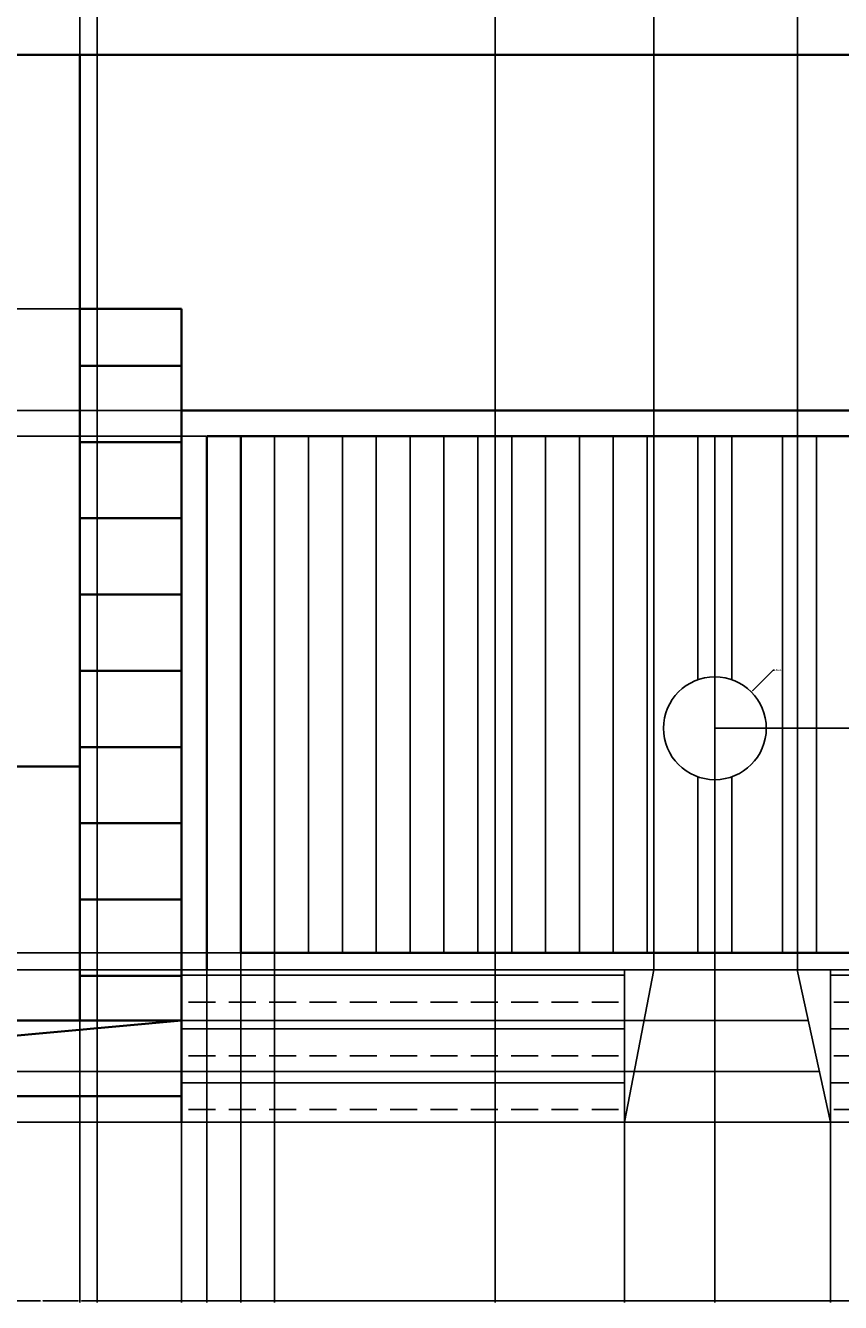
# Model space of a CAD drawing. Units: inches. Extents: x 2148 to 2587, y 1015 to 1466.
# Tile 2 of 7: x 2310 to 2406, y 1015 to 1166. Entities that reach past the tile are written whole.
import ezdxf

# ---------------------------------------------------------------- set-up
doc = ezdxf.new("R2010")
doc.units = ezdxf.units.IN
for name, color, linetype, lineweight in [('A-ANNO-DIMS', 2, 'Continuous', 18), ('A-DOOR', 3, 'Continuous', 25), ('A-ELEV', 7, 'Continuous', 35), ('A-FLOR-STRS', 2, 'Continuous', 25)]:
    doc.layers.add(name, color=color, linetype=linetype, lineweight=lineweight)
doc.styles.get("Standard").update_dxf_attribs({"font": 'arial.ttf'})
doc.dimstyles.get("Standard").update_dxf_attribs({"dimtxt": 0.18, "dimasz": 0.18, "dimexe": 0.18, "dimexo": 0.0625, "dimgap": 0.09, "dimtad": 0, "dimtih": 1, "dimtoh": 1, "dimdec": 4, "dimzin": 0, "dimdsep": 46, "dimtxsty": 'Standard', "dimcen": 0.09, "dimadec": 0, "dimazin": 0, "dimtfac": 1, "dimtdec": 4, "dimtofl": 0, "dimtmove": 0, "dimatfit": 3, "dimfxl": 1, "dimtolj": 1, "dimtzin": 0, "dimarcsym": 0})

# ---------------------------------------------------------------- blocks, each defined once
blk = doc.blocks.new('*D11')
at = {"layer": 'A-ANNO-DIMS', "color": 0, "lineweight": -2, "transparency": 16777216}
for p, q in [((2307.03, 1048.68), (2307.03, 1015.46)), ((2316.03, 1048.68), (2316.03, 1015.46)), ((2307.21, 1015.64), (2311.39, 1015.64)), ((2315.85, 1015.64), (2311.68, 1015.64))]:
    blk.add_line(p, q, dxfattribs=at)
at = {"layer": 'A-ANNO-DIMS', "color": 0, "transparency": 16777216}
for points in [[(2307.21, 1015.67), (2307.21, 1015.61), (2307.03, 1015.64)], [(2315.85, 1015.67), (2315.85, 1015.61), (2316.03, 1015.64)]]:
    blk.add_solid(points, dxfattribs=at)
at = {"layer": 'Defpoints', "color": 0, "transparency": 16777216}
for p in [(2307.03, 1048.74), (2316.03, 1048.74), (2316.03, 1015.64)]:
    blk.add_point(p, dxfattribs=at)
at = {"layer": 'A-ANNO-DIMS', "color": 0, "transparency": 16777216, "insert": (2311.53, 1015.64), "char_height": 0.18, "attachment_point": 5}
blk.add_mtext('\\A1;9', dxfattribs=at)
blk = doc.blocks.new('*D12')
at = {"layer": 'A-ANNO-DIMS', "color": 0, "lineweight": -2, "transparency": 16777216}
for p, q in [((2316.03, 1162.68), (2316.03, 1015.46)), ((2466.03, 1048.68), (2466.03, 1015.46)), ((2316.21, 1015.64), (2390.75, 1015.64)), ((2465.85, 1015.64), (2391.31, 1015.64))]:
    blk.add_line(p, q, dxfattribs=at)
at = {"layer": 'A-ANNO-DIMS', "color": 0, "transparency": 16777216}
for points in [[(2316.21, 1015.67), (2316.21, 1015.61), (2316.03, 1015.64)], [(2465.85, 1015.67), (2465.85, 1015.61), (2466.03, 1015.64)]]:
    blk.add_solid(points, dxfattribs=at)
at = {"layer": 'Defpoints', "color": 0, "transparency": 16777216}
for p in [(2316.03, 1162.74), (2466.03, 1048.74), (2466.03, 1015.64)]:
    blk.add_point(p, dxfattribs=at)
at = {"layer": 'A-ANNO-DIMS', "color": 0, "transparency": 16777216, "insert": (2391.03, 1015.64), "char_height": 0.18, "attachment_point": 5}
blk.add_mtext('\\A1;150', dxfattribs=at)
blk = doc.blocks.new('*D47')
at = {"layer": 'A-ANNO-DIMS', "color": 0, "lineweight": -2, "transparency": 16777216}
for p, q in [((2307.03, 1334.68), (2307.03, 1015.46)), ((2316.03, 1329.68), (2316.03, 1015.46)), ((2307.21, 1015.64), (2311.39, 1015.64)), ((2315.85, 1015.64), (2311.68, 1015.64))]:
    blk.add_line(p, q, dxfattribs=at)
at = {"layer": 'A-ANNO-DIMS', "color": 0, "transparency": 16777216}
for points in [[(2307.21, 1015.67), (2307.21, 1015.61), (2307.03, 1015.64)], [(2315.85, 1015.67), (2315.85, 1015.61), (2316.03, 1015.64)]]:
    blk.add_solid(points, dxfattribs=at)
at = {"layer": 'Defpoints', "color": 0, "transparency": 16777216}
for p in [(2307.03, 1334.74), (2316.03, 1329.74), (2316.03, 1015.64)]:
    blk.add_point(p, dxfattribs=at)
at = {"layer": 'A-ANNO-DIMS', "color": 0, "transparency": 16777216, "insert": (2311.53, 1015.64), "char_height": 0.18, "attachment_point": 5}
blk.add_mtext('\\A1;9', dxfattribs=at)
blk = doc.blocks.new('*D48')
at = {"layer": 'A-ANNO-DIMS', "color": 0, "lineweight": -2, "transparency": 16777216}
for p, q in [((2316.03, 1329.68), (2316.03, 1015.46)), ((2318.08, 1174.68), (2318.08, 1015.46)), ((2316.21, 1015.64), (2316.73, 1015.64)), ((2317.9, 1015.64), (2317.38, 1015.64))]:
    blk.add_line(p, q, dxfattribs=at)
at = {"layer": 'A-ANNO-DIMS', "color": 0, "transparency": 16777216}
for points in [[(2316.21, 1015.67), (2316.21, 1015.61), (2316.03, 1015.64)], [(2317.9, 1015.67), (2317.9, 1015.61), (2318.08, 1015.64)]]:
    blk.add_solid(points, dxfattribs=at)
at = {"layer": 'Defpoints', "color": 0, "transparency": 16777216}
for p in [(2316.03, 1329.74), (2318.08, 1174.74), (2318.08, 1015.64)]:
    blk.add_point(p, dxfattribs=at)
at = {"layer": 'A-ANNO-DIMS', "color": 0, "transparency": 16777216, "insert": (2317.06, 1015.64), "char_height": 0.18, "attachment_point": 5}
blk.add_mtext('\\A1;2.05', dxfattribs=at)
blk = doc.blocks.new('*D49')
at = {"layer": 'A-ANNO-DIMS', "color": 0, "lineweight": -2, "transparency": 16777216}
for p, q in [((2318.08, 1174.68), (2318.08, 1015.46)), ((2365.07, 1174.68), (2365.07, 1015.46)), ((2318.26, 1015.64), (2341.18, 1015.64)), ((2364.89, 1015.64), (2341.97, 1015.64))]:
    blk.add_line(p, q, dxfattribs=at)
at = {"layer": 'A-ANNO-DIMS', "color": 0, "transparency": 16777216}
for points in [[(2318.26, 1015.67), (2318.26, 1015.61), (2318.08, 1015.64)], [(2364.89, 1015.67), (2364.89, 1015.61), (2365.07, 1015.64)]]:
    blk.add_solid(points, dxfattribs=at)
at = {"layer": 'Defpoints', "color": 0, "transparency": 16777216}
for p in [(2318.08, 1174.74), (2365.07, 1174.74), (2365.07, 1015.64)]:
    blk.add_point(p, dxfattribs=at)
at = {"layer": 'A-ANNO-DIMS', "color": 0, "transparency": 16777216, "insert": (2341.58, 1015.64), "char_height": 0.18, "attachment_point": 5}
blk.add_mtext('\\A1;46.99', dxfattribs=at)
blk = doc.blocks.new('*D50')
at = {"layer": 'A-ANNO-DIMS', "color": 0, "lineweight": -2, "transparency": 16777216}
for p, q in [((2365.07, 1174.68), (2365.07, 1015.46)), ((2412.06, 1174.68), (2412.06, 1015.46)), ((2365.25, 1015.64), (2388.16, 1015.64)), ((2411.88, 1015.64), (2388.96, 1015.64))]:
    blk.add_line(p, q, dxfattribs=at)
at = {"layer": 'A-ANNO-DIMS', "color": 0, "transparency": 16777216}
for points in [[(2365.25, 1015.67), (2365.25, 1015.61), (2365.07, 1015.64)], [(2411.88, 1015.67), (2411.88, 1015.61), (2412.06, 1015.64)]]:
    blk.add_solid(points, dxfattribs=at)
at = {"layer": 'Defpoints', "color": 0, "transparency": 16777216}
for p in [(2365.07, 1174.74), (2412.06, 1174.74), (2412.06, 1015.64)]:
    blk.add_point(p, dxfattribs=at)
at = {"layer": 'A-ANNO-DIMS', "color": 0, "transparency": 16777216, "insert": (2388.56, 1015.64), "char_height": 0.18, "attachment_point": 5}
blk.add_mtext('\\A1;46.99', dxfattribs=at)
blk = doc.blocks.new('*D98')
at = {"layer": 'A-ANNO-DIMS', "color": 0, "lineweight": -2, "transparency": 16777216}
for p, q in [((2383.84, 1054.81), (2383.84, 1466.02)), ((2384.02, 1465.84), (2391.92, 1465.84)), ((2400.59, 1465.84), (2392.69, 1465.84)), ((2400.77, 1054.81), (2400.77, 1466.02))]:
    blk.add_line(p, q, dxfattribs=at)
at = {"layer": 'A-ANNO-DIMS', "color": 0, "transparency": 16777216}
for points in [[(2384.02, 1465.87), (2384.02, 1465.81), (2383.84, 1465.84)], [(2400.59, 1465.87), (2400.59, 1465.81), (2400.77, 1465.84)]]:
    blk.add_solid(points, dxfattribs=at)
at = {"layer": 'Defpoints', "color": 0, "transparency": 16777216}
for p in [(2400.77, 1465.84), (2383.84, 1054.74), (2400.77, 1054.74)]:
    blk.add_point(p, dxfattribs=at)
at = {"layer": 'A-ANNO-DIMS', "color": 0, "transparency": 16777216, "insert": (2392.3, 1465.84), "char_height": 0.18, "attachment_point": 5}
blk.add_mtext('\\A1;16.93', dxfattribs=at)
blk = doc.blocks.new('*D99')
at = {"layer": 'A-ANNO-DIMS', "color": 0, "lineweight": -2, "transparency": 16777216}
for p, q in [((2316.03, 1048.68), (2316.03, 1015.46)), ((2328.03, 1036.68), (2328.03, 1015.46)), ((2316.21, 1015.64), (2321.82, 1015.64)), ((2327.85, 1015.64), (2322.24, 1015.64))]:
    blk.add_line(p, q, dxfattribs=at)
at = {"layer": 'A-ANNO-DIMS', "color": 0, "transparency": 16777216}
for points in [[(2316.21, 1015.67), (2316.21, 1015.61), (2316.03, 1015.64)], [(2327.85, 1015.67), (2327.85, 1015.61), (2328.03, 1015.64)]]:
    blk.add_solid(points, dxfattribs=at)
at = {"layer": 'Defpoints', "color": 0, "transparency": 16777216}
for p in [(2316.03, 1048.74), (2328.03, 1036.74), (2328.03, 1015.64)]:
    blk.add_point(p, dxfattribs=at)
at = {"layer": 'A-ANNO-DIMS', "color": 0, "transparency": 16777216, "insert": (2322.03, 1015.64), "char_height": 0.18, "attachment_point": 5}
blk.add_mtext('\\A1;12', dxfattribs=at)
blk = doc.blocks.new('*D100')
at = {"layer": 'A-ANNO-DIMS', "color": 0, "lineweight": -2, "transparency": 16777216}
for p, q in [((2331.03, 1117.68), (2331.03, 1015.46)), ((2328.03, 1036.68), (2328.03, 1015.46)), ((2328.21, 1015.64), (2329.39, 1015.64)), ((2330.85, 1015.64), (2329.68, 1015.64))]:
    blk.add_line(p, q, dxfattribs=at)
at = {"layer": 'A-ANNO-DIMS', "color": 0, "transparency": 16777216}
for points in [[(2328.21, 1015.67), (2328.21, 1015.61), (2328.03, 1015.64)], [(2330.85, 1015.67), (2330.85, 1015.61), (2331.03, 1015.64)]]:
    blk.add_solid(points, dxfattribs=at)
at = {"layer": 'Defpoints', "color": 0, "transparency": 16777216}
for p in [(2331.03, 1117.74), (2328.03, 1036.74), (2331.03, 1015.64)]:
    blk.add_point(p, dxfattribs=at)
at = {"layer": 'A-ANNO-DIMS', "color": 0, "transparency": 16777216, "insert": (2329.53, 1015.64), "char_height": 0.18, "attachment_point": 5}
blk.add_mtext('\\A1;3', dxfattribs=at)
blk = doc.blocks.new('*D101')
at = {"layer": 'A-ANNO-DIMS', "color": 0, "lineweight": -2, "transparency": 16777216}
for p, q in [((2331.03, 1117.68), (2331.03, 1015.46)), ((2335.03, 1056.68), (2335.03, 1015.46)), ((2331.21, 1015.64), (2332.88, 1015.64)), ((2334.85, 1015.64), (2333.19, 1015.64))]:
    blk.add_line(p, q, dxfattribs=at)
at = {"layer": 'A-ANNO-DIMS', "color": 0, "transparency": 16777216}
for points in [[(2331.21, 1015.67), (2331.21, 1015.61), (2331.03, 1015.64)], [(2334.85, 1015.67), (2334.85, 1015.61), (2335.03, 1015.64)]]:
    blk.add_solid(points, dxfattribs=at)
at = {"layer": 'Defpoints', "color": 0, "transparency": 16777216}
for p in [(2331.03, 1117.74), (2335.03, 1056.74), (2335.03, 1015.64)]:
    blk.add_point(p, dxfattribs=at)
at = {"layer": 'A-ANNO-DIMS', "color": 0, "transparency": 16777216, "insert": (2333.03, 1015.64), "char_height": 0.18, "attachment_point": 5}
blk.add_mtext('\\A1;4', dxfattribs=at)
blk = doc.blocks.new('*D102')
at = {"layer": 'A-ANNO-DIMS', "color": 0, "lineweight": -2, "transparency": 16777216}
for p, q in [((2335.03, 1056.68), (2335.03, 1015.46)), ((2339.03, 1056.68), (2339.03, 1015.46)), ((2335.21, 1015.64), (2336.88, 1015.64)), ((2338.85, 1015.64), (2337.19, 1015.64))]:
    blk.add_line(p, q, dxfattribs=at)
at = {"layer": 'A-ANNO-DIMS', "color": 0, "transparency": 16777216}
for points in [[(2335.21, 1015.67), (2335.21, 1015.61), (2335.03, 1015.64)], [(2338.85, 1015.67), (2338.85, 1015.61), (2339.03, 1015.64)]]:
    blk.add_solid(points, dxfattribs=at)
at = {"layer": 'Defpoints', "color": 0, "transparency": 16777216}
for p in [(2335.03, 1056.74), (2339.03, 1056.74), (2339.03, 1015.64)]:
    blk.add_point(p, dxfattribs=at)
at = {"layer": 'A-ANNO-DIMS', "color": 0, "transparency": 16777216, "insert": (2337.03, 1015.64), "char_height": 0.18, "attachment_point": 5}
blk.add_mtext('\\A1;4', dxfattribs=at)
blk = doc.blocks.new('*D103')
at = {"layer": 'A-ANNO-DIMS', "color": 0, "lineweight": -2, "transparency": 16777216}
for p, q in [((2339.03, 1056.68), (2339.03, 1015.46)), ((2380.36, 1036.68), (2380.36, 1015.46)), ((2339.21, 1015.64), (2359.3, 1015.64)), ((2380.18, 1015.64), (2360.1, 1015.64))]:
    blk.add_line(p, q, dxfattribs=at)
at = {"layer": 'A-ANNO-DIMS', "color": 0, "transparency": 16777216}
for points in [[(2339.21, 1015.67), (2339.21, 1015.61), (2339.03, 1015.64)], [(2380.18, 1015.67), (2380.18, 1015.61), (2380.36, 1015.64)]]:
    blk.add_solid(points, dxfattribs=at)
at = {"layer": 'Defpoints', "color": 0, "transparency": 16777216}
for p in [(2339.03, 1056.74), (2380.36, 1036.74), (2380.36, 1015.64)]:
    blk.add_point(p, dxfattribs=at)
at = {"layer": 'A-ANNO-DIMS', "color": 0, "transparency": 16777216, "insert": (2359.7, 1015.64), "char_height": 0.18, "attachment_point": 5}
blk.add_mtext('\\A1;41.33', dxfattribs=at)
blk = doc.blocks.new('*D104')
at = {"layer": 'A-ANNO-DIMS', "color": 0, "lineweight": -2, "transparency": 16777216}
for p, q in [((2391.03, 1083.18), (2391.03, 1015.46)), ((2380.36, 1036.68), (2380.36, 1015.46)), ((2380.54, 1015.64), (2385.31, 1015.64)), ((2390.85, 1015.64), (2386.08, 1015.64))]:
    blk.add_line(p, q, dxfattribs=at)
at = {"layer": 'A-ANNO-DIMS', "color": 0, "transparency": 16777216}
for points in [[(2380.54, 1015.67), (2380.54, 1015.61), (2380.36, 1015.64)], [(2390.85, 1015.67), (2390.85, 1015.61), (2391.03, 1015.64)]]:
    blk.add_solid(points, dxfattribs=at)
at = {"layer": 'Defpoints', "color": 0, "transparency": 16777216}
for p in [(2391.03, 1083.24), (2380.36, 1036.74), (2391.03, 1015.64)]:
    blk.add_point(p, dxfattribs=at)
at = {"layer": 'A-ANNO-DIMS', "color": 0, "transparency": 16777216, "insert": (2385.7, 1015.64), "char_height": 0.18, "attachment_point": 5}
blk.add_mtext('\\A1;10.67', dxfattribs=at)
blk = doc.blocks.new('*D105')
at = {"layer": 'A-ANNO-DIMS', "color": 0, "lineweight": -2, "transparency": 16777216}
for p, q in [((2391.03, 1083.18), (2391.03, 1015.46)), ((2404.7, 1036.68), (2404.7, 1015.46)), ((2391.21, 1015.64), (2397.48, 1015.64)), ((2404.52, 1015.64), (2398.25, 1015.64))]:
    blk.add_line(p, q, dxfattribs=at)
at = {"layer": 'A-ANNO-DIMS', "color": 0, "transparency": 16777216}
for points in [[(2391.21, 1015.67), (2391.21, 1015.61), (2391.03, 1015.64)], [(2404.52, 1015.67), (2404.52, 1015.61), (2404.7, 1015.64)]]:
    blk.add_solid(points, dxfattribs=at)
at = {"layer": 'Defpoints', "color": 0, "transparency": 16777216}
for p in [(2391.03, 1083.24), (2404.7, 1036.74), (2404.7, 1015.64)]:
    blk.add_point(p, dxfattribs=at)
at = {"layer": 'A-ANNO-DIMS', "color": 0, "transparency": 16777216, "insert": (2397.86, 1015.64), "char_height": 0.18, "attachment_point": 5}
blk.add_mtext('\\A1;13.66', dxfattribs=at)
blk = doc.blocks.new('*D106')
at = {"layer": 'A-ANNO-DIMS', "color": 0, "lineweight": -2, "transparency": 16777216}
for p, q in [((2447.03, 1056.68), (2447.03, 1015.46)), ((2404.7, 1036.68), (2404.7, 1015.46)), ((2404.88, 1015.64), (2425.47, 1015.64)), ((2446.85, 1015.64), (2426.26, 1015.64))]:
    blk.add_line(p, q, dxfattribs=at)
at = {"layer": 'A-ANNO-DIMS', "color": 0, "transparency": 16777216}
for points in [[(2404.88, 1015.67), (2404.88, 1015.61), (2404.7, 1015.64)], [(2446.85, 1015.67), (2446.85, 1015.61), (2447.03, 1015.64)]]:
    blk.add_solid(points, dxfattribs=at)
at = {"layer": 'Defpoints', "color": 0, "transparency": 16777216}
for p in [(2447.03, 1056.74), (2404.7, 1036.74), (2447.03, 1015.64)]:
    blk.add_point(p, dxfattribs=at)
at = {"layer": 'A-ANNO-DIMS', "color": 0, "transparency": 16777216, "insert": (2425.86, 1015.64), "char_height": 0.18, "attachment_point": 5}
blk.add_mtext('\\A1;42.34', dxfattribs=at)
blk = doc.blocks.new('*D110')
at = {"layer": 'A-ANNO-DIMS', "color": 0, "lineweight": -2, "transparency": 16777216}
for p, q in [((2327.97, 1039.82), (2147.75, 1039.82)), ((2147.93, 1039.64), (2147.93, 1038.46)), ((2147.93, 1036.92), (2147.93, 1038.1)), ((2327.97, 1036.74), (2147.75, 1036.74))]:
    blk.add_line(p, q, dxfattribs=at)
at = {"layer": 'A-ANNO-DIMS', "color": 0, "transparency": 16777216}
for points in [[(2147.9, 1039.64), (2147.96, 1039.64), (2147.93, 1039.82)], [(2147.9, 1036.92), (2147.96, 1036.92), (2147.93, 1036.74)]]:
    blk.add_solid(points, dxfattribs=at)
at = {"layer": 'Defpoints', "color": 0, "transparency": 16777216}
for p in [(2147.93, 1039.82), (2328.03, 1039.82), (2328.03, 1036.74)]:
    blk.add_point(p, dxfattribs=at)
at = {"layer": 'A-ANNO-DIMS', "color": 0, "transparency": 16777216, "insert": (2147.93, 1038.28), "char_height": 0.18, "attachment_point": 5}
blk.add_mtext('\\A1;3.07', dxfattribs=at)
blk = doc.blocks.new('*D111')
at = {"layer": 'A-ANNO-DIMS', "color": 0, "lineweight": -2, "transparency": 16777216}
for p, q in [((2327.97, 1048.74), (2147.75, 1048.74)), ((2147.93, 1048.56), (2147.93, 1044.46)), ((2147.93, 1040), (2147.93, 1044.1)), ((2327.97, 1039.82), (2147.75, 1039.82))]:
    blk.add_line(p, q, dxfattribs=at)
at = {"layer": 'A-ANNO-DIMS', "color": 0, "transparency": 16777216}
for points in [[(2147.9, 1048.56), (2147.96, 1048.56), (2147.93, 1048.74)], [(2147.9, 1040), (2147.96, 1040), (2147.93, 1039.82)]]:
    blk.add_solid(points, dxfattribs=at)
at = {"layer": 'Defpoints', "color": 0, "transparency": 16777216}
for p in [(2147.93, 1048.74), (2328.03, 1048.74), (2328.03, 1039.82)]:
    blk.add_point(p, dxfattribs=at)
at = {"layer": 'A-ANNO-DIMS', "color": 0, "transparency": 16777216, "insert": (2147.93, 1044.28), "char_height": 0.18, "attachment_point": 5}
blk.add_mtext('\\A1;8.925', dxfattribs=at)
blk = doc.blocks.new('*D112')
at = {"layer": 'A-ANNO-DIMS', "color": 0, "lineweight": -2, "transparency": 16777216}
for p, q in [((2327.97, 1054.74), (2147.75, 1054.74)), ((2147.93, 1054.56), (2147.93, 1051.92)), ((2147.93, 1048.92), (2147.93, 1051.56)), ((2327.97, 1048.74), (2147.75, 1048.74))]:
    blk.add_line(p, q, dxfattribs=at)
at = {"layer": 'A-ANNO-DIMS', "color": 0, "transparency": 16777216}
for points in [[(2147.9, 1054.56), (2147.96, 1054.56), (2147.93, 1054.74)], [(2147.9, 1048.92), (2147.96, 1048.92), (2147.93, 1048.74)]]:
    blk.add_solid(points, dxfattribs=at)
at = {"layer": 'Defpoints', "color": 0, "transparency": 16777216}
for p in [(2147.93, 1054.74), (2328.03, 1054.74), (2328.03, 1048.74)]:
    blk.add_point(p, dxfattribs=at)
at = {"layer": 'A-ANNO-DIMS', "color": 0, "transparency": 16777216, "insert": (2147.93, 1051.74), "char_height": 0.18, "attachment_point": 5}
blk.add_mtext('\\A1;6', dxfattribs=at)
blk = doc.blocks.new('*D113')
at = {"layer": 'A-ANNO-DIMS', "color": 0, "lineweight": -2, "transparency": 16777216}
for p, q in [((2334.97, 1056.74), (2147.75, 1056.74)), ((2147.93, 1056.56), (2147.93, 1055.92)), ((2147.93, 1054.92), (2147.93, 1055.56)), ((2327.97, 1054.74), (2147.75, 1054.74))]:
    blk.add_line(p, q, dxfattribs=at)
at = {"layer": 'A-ANNO-DIMS', "color": 0, "transparency": 16777216}
for points in [[(2147.9, 1056.56), (2147.96, 1056.56), (2147.93, 1056.74)], [(2147.9, 1054.92), (2147.96, 1054.92), (2147.93, 1054.74)]]:
    blk.add_solid(points, dxfattribs=at)
at = {"layer": 'Defpoints', "color": 0, "transparency": 16777216}
for p in [(2147.93, 1056.74), (2335.03, 1056.74), (2328.03, 1054.74)]:
    blk.add_point(p, dxfattribs=at)
at = {"layer": 'A-ANNO-DIMS', "color": 0, "transparency": 16777216, "insert": (2147.93, 1055.74), "char_height": 0.18, "attachment_point": 5}
blk.add_mtext('\\A1;2', dxfattribs=at)
blk = doc.blocks.new('*D114')
at = {"layer": 'A-ANNO-DIMS', "color": 0, "lineweight": -2, "transparency": 16777216}
for p, q in [((2330.97, 1117.74), (2147.75, 1117.74)), ((2147.93, 1117.56), (2147.93, 1087.42)), ((2147.93, 1056.92), (2147.93, 1087.06)), ((2334.97, 1056.74), (2147.75, 1056.74))]:
    blk.add_line(p, q, dxfattribs=at)
at = {"layer": 'A-ANNO-DIMS', "color": 0, "transparency": 16777216}
for points in [[(2147.9, 1117.56), (2147.96, 1117.56), (2147.93, 1117.74)], [(2147.9, 1056.92), (2147.96, 1056.92), (2147.93, 1056.74)]]:
    blk.add_solid(points, dxfattribs=at)
at = {"layer": 'Defpoints', "color": 0, "transparency": 16777216}
for p in [(2147.93, 1117.74), (2331.03, 1117.74), (2335.03, 1056.74)]:
    blk.add_point(p, dxfattribs=at)
at = {"layer": 'A-ANNO-DIMS', "color": 0, "transparency": 16777216, "insert": (2147.93, 1087.24), "char_height": 0.18, "attachment_point": 5}
blk.add_mtext('\\A1;61', dxfattribs=at)
blk = doc.blocks.new('*D115')
at = {"layer": 'A-ANNO-DIMS', "color": 0, "lineweight": -2, "transparency": 16777216}
for p, q in [((2327.97, 1120.74), (2147.75, 1120.74)), ((2147.93, 1120.56), (2147.93, 1119.42)), ((2147.93, 1117.92), (2147.93, 1119.06)), ((2330.97, 1117.74), (2147.75, 1117.74))]:
    blk.add_line(p, q, dxfattribs=at)
at = {"layer": 'A-ANNO-DIMS', "color": 0, "transparency": 16777216}
for points in [[(2147.9, 1120.56), (2147.96, 1120.56), (2147.93, 1120.74)], [(2147.9, 1117.92), (2147.96, 1117.92), (2147.93, 1117.74)]]:
    blk.add_solid(points, dxfattribs=at)
at = {"layer": 'Defpoints', "color": 0, "transparency": 16777216}
for p in [(2147.93, 1120.74), (2328.03, 1120.74), (2331.03, 1117.74)]:
    blk.add_point(p, dxfattribs=at)
at = {"layer": 'A-ANNO-DIMS', "color": 0, "transparency": 16777216, "insert": (2147.93, 1119.24), "char_height": 0.18, "attachment_point": 5}
blk.add_mtext('\\A1;3', dxfattribs=at)
blk = doc.blocks.new('*D116')
at = {"layer": 'A-ANNO-DIMS', "color": 0, "lineweight": -2, "transparency": 16777216}
for p, q in [((2327.97, 1132.74), (2147.75, 1132.74)), ((2147.93, 1132.56), (2147.93, 1126.92)), ((2147.93, 1120.92), (2147.93, 1126.56)), ((2327.97, 1120.74), (2147.75, 1120.74))]:
    blk.add_line(p, q, dxfattribs=at)
at = {"layer": 'A-ANNO-DIMS', "color": 0, "transparency": 16777216}
for points in [[(2147.9, 1132.56), (2147.96, 1132.56), (2147.93, 1132.74)], [(2147.9, 1120.92), (2147.96, 1120.92), (2147.93, 1120.74)]]:
    blk.add_solid(points, dxfattribs=at)
at = {"layer": 'Defpoints', "color": 0, "transparency": 16777216}
for p in [(2147.93, 1132.74), (2328.03, 1132.74), (2328.03, 1120.74)]:
    blk.add_point(p, dxfattribs=at)
at = {"layer": 'A-ANNO-DIMS', "color": 0, "transparency": 16777216, "insert": (2147.93, 1126.74), "char_height": 0.18, "attachment_point": 5}
blk.add_mtext('\\A1;12', dxfattribs=at)
blk = doc.blocks.new('*D117')
at = {"layer": 'A-ANNO-DIMS', "color": 0, "lineweight": -2, "transparency": 16777216}
for p, q in [((2403.32, 1042.74), (2147.75, 1042.74)), ((2147.93, 1042.56), (2147.93, 1039.92)), ((2147.93, 1036.92), (2147.93, 1039.56)), ((2404.63, 1036.74), (2147.75, 1036.74))]:
    blk.add_line(p, q, dxfattribs=at)
at = {"layer": 'A-ANNO-DIMS', "color": 0, "transparency": 16777216}
for points in [[(2147.9, 1042.56), (2147.96, 1042.56), (2147.93, 1042.74)], [(2147.9, 1036.92), (2147.96, 1036.92), (2147.93, 1036.74)]]:
    blk.add_solid(points, dxfattribs=at)
at = {"layer": 'Defpoints', "color": 0, "transparency": 16777216}
for p in [(2147.93, 1042.74), (2403.39, 1042.74), (2404.7, 1036.74)]:
    blk.add_point(p, dxfattribs=at)
at = {"layer": 'A-ANNO-DIMS', "color": 0, "transparency": 16777216, "insert": (2147.93, 1039.74), "char_height": 0.18, "attachment_point": 5}
blk.add_mtext('\\A1;6', dxfattribs=at)
blk = doc.blocks.new('*D118')
at = {"layer": 'A-ANNO-DIMS', "color": 0, "lineweight": -2, "transparency": 16777216}
for p, q in [((2402.02, 1048.74), (2147.75, 1048.74)), ((2147.93, 1048.56), (2147.93, 1045.92)), ((2147.93, 1042.92), (2147.93, 1045.56)), ((2403.32, 1042.74), (2147.75, 1042.74))]:
    blk.add_line(p, q, dxfattribs=at)
at = {"layer": 'A-ANNO-DIMS', "color": 0, "transparency": 16777216}
for points in [[(2147.9, 1048.56), (2147.96, 1048.56), (2147.93, 1048.74)], [(2147.9, 1042.92), (2147.96, 1042.92), (2147.93, 1042.74)]]:
    blk.add_solid(points, dxfattribs=at)
at = {"layer": 'Defpoints', "color": 0, "transparency": 16777216}
for p in [(2147.93, 1048.74), (2402.08, 1048.74), (2403.39, 1042.74)]:
    blk.add_point(p, dxfattribs=at)
at = {"layer": 'A-ANNO-DIMS', "color": 0, "transparency": 16777216, "insert": (2147.93, 1045.74), "char_height": 0.18, "attachment_point": 5}
blk.add_mtext('\\A1;6', dxfattribs=at)
blk = doc.blocks.new('*D119')
at = {"layer": 'A-ANNO-DIMS', "color": 0, "lineweight": -2, "transparency": 16777216}
for p, q in [((2400.71, 1054.74), (2147.75, 1054.74)), ((2147.93, 1054.56), (2147.93, 1051.92)), ((2147.93, 1048.92), (2147.93, 1051.56)), ((2402.02, 1048.74), (2147.75, 1048.74))]:
    blk.add_line(p, q, dxfattribs=at)
at = {"layer": 'A-ANNO-DIMS', "color": 0, "transparency": 16777216}
for points in [[(2147.9, 1054.56), (2147.96, 1054.56), (2147.93, 1054.74)], [(2147.9, 1048.92), (2147.96, 1048.92), (2147.93, 1048.74)]]:
    blk.add_solid(points, dxfattribs=at)
at = {"layer": 'Defpoints', "color": 0, "transparency": 16777216}
for p in [(2147.93, 1054.74), (2400.77, 1054.74), (2402.08, 1048.74)]:
    blk.add_point(p, dxfattribs=at)
at = {"layer": 'A-ANNO-DIMS', "color": 0, "transparency": 16777216, "insert": (2147.93, 1051.74), "char_height": 0.18, "attachment_point": 5}
blk.add_mtext('\\A1;6', dxfattribs=at)
blk = doc.blocks.new('*D120')
at = {"layer": 'A-ANNO-DIMS', "color": 0, "lineweight": -2, "transparency": 16777216}
for p, q in [((2391.1, 1083.24), (2586.31, 1083.24)), ((2586.13, 1083.06), (2586.13, 1069.17)), ((2586.13, 1054.92), (2586.13, 1068.81)), ((2454.1, 1054.74), (2586.31, 1054.74))]:
    blk.add_line(p, q, dxfattribs=at)
at = {"layer": 'A-ANNO-DIMS', "color": 0, "transparency": 16777216}
for points in [[(2586.1, 1083.06), (2586.16, 1083.06), (2586.13, 1083.24)], [(2586.1, 1054.92), (2586.16, 1054.92), (2586.13, 1054.74)]]:
    blk.add_solid(points, dxfattribs=at)
at = {"layer": 'Defpoints', "color": 0, "transparency": 16777216}
for p in [(2391.03, 1083.24), (2586.13, 1083.24), (2454.03, 1054.74)]:
    blk.add_point(p, dxfattribs=at)
at = {"layer": 'A-ANNO-DIMS', "color": 0, "transparency": 16777216, "insert": (2586.13, 1068.99), "char_height": 0.18, "attachment_point": 5}
blk.add_mtext('\\A1;28.5', dxfattribs=at)
blk = doc.blocks.new('*D123')
at = {"layer": 'A-ANNO-DIMS', "color": 0, "lineweight": -2, "transparency": 16777216}
for p, q in [((2397.91, 1090.1), (2395.46, 1087.66)), ((2398.09, 1090.1), (2397.91, 1090.1)), ((2390.94, 1083.24), (2391.12, 1083.24)), ((2391.03, 1083.15), (2391.03, 1083.33))]:
    blk.add_line(p, q, dxfattribs=at)
at = {"layer": 'A-ANNO-DIMS', "color": 0, "transparency": 16777216}
blk.add_solid([(2395.44, 1087.68), (2395.48, 1087.64), (2395.33, 1087.53)], dxfattribs=at)
at = {"layer": 'Defpoints', "color": 0, "transparency": 16777216}
for p in [(2395.33, 1087.53), (2386.74, 1078.96)]:
    blk.add_point(p, dxfattribs=at)
at = {"layer": 'A-ANNO-DIMS', "color": 0, "transparency": 16777216, "insert": (2398.65, 1090.1), "char_height": 0.18, "attachment_point": 5}
blk.add_mtext('\\A1;∅12.138', dxfattribs=at)

msp = doc.modelspace()

# ---------------------------------------------------------------- hatches: boundary and pattern name
at = {"layer": 'A-FLOR-STRS'}
h = msp.add_hatch(dxfattribs=at)
h.set_pattern_fill('BRASS', color=256)
h.paths.add_polyline_path([(2380.364, 1054.7427), (2331.0343, 1054.7427), (2328.0343, 1054.7427), (2328.0343, 1036.7427), (2380.364, 1036.7427)])
h.paths.add_polyline_path([(2454.0343, 1054.7427), (2451.0343, 1054.7427), (2404.6955, 1054.7427), (2404.6955, 1036.7427), (2454.0343, 1036.7427)])

# ---------------------------------------------------------------- linework, layer by layer
at = {"layer": 'A-DOOR'}
for p, q in [((2339.0343, 1056.7427), (2339.0343, 1117.7427)), ((2343.0343, 1056.7427), (2343.0343, 1117.7427)), ((2347.0343, 1056.7427), (2347.0343, 1117.7427)), ((2351.0343, 1056.7427), (2351.0343, 1117.7427)), ((2355.0343, 1056.7427), (2355.0343, 1117.7427)), ((2359.0343, 1056.7427), (2359.0343, 1117.7427)), ((2363.0343, 1056.7427), (2363.0343, 1117.7427)), ((2367.0343, 1056.7427), (2367.0343, 1117.7427)), ((2371.0343, 1056.7427), (2371.0343, 1117.7427)), ((2375.0343, 1056.7427), (2375.0343, 1117.7427)), ((2379.0343, 1056.7427), (2379.0343, 1117.7427)), ((2383.0343, 1056.7427), (2383.0343, 1117.7427)), ((2389.0343, 1117.7427), (2389.0343, 1088.9725)), ((2391.0343, 1117.7427), (2391.0343, 1056.7427)), ((2393.0343, 1117.7427), (2393.0343, 1088.9725)), ((2399.0343, 1056.7427), (2399.0343, 1117.7427)), ((2403.0343, 1056.7427), (2403.0343, 1117.7427)), ((2389.0343, 1077.5128), (2389.0343, 1056.7427)), ((2393.0343, 1077.5128), (2393.0343, 1056.7427))]:
    msp.add_line(p, q, dxfattribs=at)
msp.add_circle((2391.0343, 1083.2427), 6.0689, dxfattribs=at)
at = {"layer": 'A-ELEV'}
for p, q in [((2547.0343, 1162.7427), (2187.0343, 1162.7427)), ((2316.0343, 1048.7427), (2316.0343, 1162.7427)), ((2328.0343, 1132.7427), (2316.0343, 1132.7427)), ((2328.0343, 1048.7427), (2328.0343, 1132.7427)), ((2316.0343, 1126.0305), (2328.0343, 1126.0305)), ((2454.0343, 1120.7427), (2328.0343, 1120.7427)), ((2316.0343, 1117.0305), (2328.0343, 1117.0305)), ((2451.0343, 1117.7427), (2331.0343, 1117.7427)), ((2331.0343, 1054.7427), (2331.0343, 1117.7427)), ((2335.0343, 1056.7427), (2335.0343, 1117.7427)), ((2316.0343, 1108.0305), (2328.0343, 1108.0305)), ((2316.0343, 1099.0305), (2328.0343, 1099.0305)), ((2316.0343, 1090.0305), (2328.0343, 1090.0305)), ((2316.0343, 1081.0305), (2328.0343, 1081.0305)), ((2316.0343, 1078.7427), (2307.0343, 1078.7427)), ((2316.0343, 1072.0305), (2328.0343, 1072.0305)), ((2316.0343, 1063.0305), (2328.0343, 1063.0305)), ((2328.0343, 1063.0305), (2328.0343, 1036.7427)), ((2391.0343, 1056.7427), (2335.0343, 1056.7427)), ((2447.0343, 1056.7427), (2391.0343, 1056.7427)), ((2316.0343, 1054.0305), (2328.0343, 1054.0305)), ((2328.0343, 1048.7427), (2187.0343, 1048.7427)), ((2328.0343, 1048.7427), (2229.9391, 1039.8173)), ((2328.0343, 1039.8173), (2187.0343, 1039.8173))]:
    msp.add_line(p, q, dxfattribs=at)
at = {"layer": 'A-FLOR-STRS'}
for p, q in [((2331.0343, 1054.7427), (2328.0343, 1054.7427)), ((2391.0343, 1054.7427), (2331.0343, 1054.7427)), ((2380.364, 1036.7427), (2380.364, 1054.7427)), ((2380.364, 1036.7427), (2383.84, 1054.7427)), ((2451.0343, 1054.7427), (2391.0343, 1054.7427)), ((2404.6955, 1036.7427), (2400.7695, 1054.7427)), ((2404.6955, 1036.7427), (2404.6955, 1054.7427)), ((2402.0782, 1048.7427), (2382.6813, 1048.7427)), ((2403.3868, 1042.7427), (2381.5227, 1042.7427)), ((2454.0343, 1036.7427), (2328.0343, 1036.7427))]:
    msp.add_line(p, q, dxfattribs=at)

# ---------------------------------------------------------------- dimensions: what is measured, and where the dimension line sits
at = {"layer": 'A-ANNO-DIMS'}
for base, p1, p2, override, picture, middle in [((2400.7695, 1465.8427), (2383.84, 1054.7427), (2400.7695, 1054.7427), {"dimdec": 2, "dimlfac": 1, "dimrnd": 0, "dimzin": 0, "dimdsep": 46, "dimlunit": 2}, '*D98', (2392.3048, 1465.8427)), ((2316.0343, 1015.6427), (2307.0343, 1334.7427), (2316.0343, 1329.7427), {"dimdec": 0, "dimlfac": 1, "dimrnd": 0, "dimzin": 0, "dimdsep": 46, "dimlunit": 2}, '*D47', (2311.5343, 1015.6427)), ((2318.0835, 1015.6427), (2316.0343, 1329.7427), (2318.0835, 1174.7427), {"dimdec": 2, "dimlfac": 1, "dimrnd": 0, "dimzin": 0, "dimdsep": 46, "dimlunit": 2}, '*D48', (2317.0589, 1015.6427)), ((2365.0695, 1015.6427), (2318.0835, 1174.7427), (2365.0695, 1174.7427), {"dimdec": 2, "dimlfac": 1, "dimrnd": 0, "dimzin": 0, "dimdsep": 46, "dimlunit": 2}, '*D49', (2341.5765, 1015.6427)), ((2412.0554, 1015.6427), (2365.0695, 1174.7427), (2412.0554, 1174.7427), {"dimdec": 2, "dimlfac": 1, "dimrnd": 0, "dimzin": 0, "dimdsep": 46, "dimlunit": 2}, '*D50', (2388.5624, 1015.6427)), ((2466.0343, 1015.6427), (2316.0343, 1162.7427), (2466.0343, 1048.7427), {"dimdec": 0, "dimlfac": 1, "dimrnd": 0, "dimzin": 0, "dimdsep": 46, "dimlunit": 2}, '*D12', (2391.0343, 1015.6427)), ((2331.0343, 1015.6427), (2328.0343, 1036.7427), (2331.0343, 1117.7427), {"dimdec": 0, "dimlfac": 1, "dimrnd": 0, "dimzin": 0, "dimdsep": 46, "dimlunit": 2}, '*D100', (2329.5343, 1015.6427)), ((2335.0343, 1015.6427), (2331.0343, 1117.7427), (2335.0343, 1056.7427), {"dimdec": 0, "dimlfac": 1, "dimrnd": 0, "dimzin": 0, "dimdsep": 46, "dimlunit": 2}, '*D101', (2333.0343, 1015.6427)), ((2391.0343, 1015.6427), (2380.364, 1036.7427), (2391.0343, 1083.2427), {"dimdec": 2, "dimlfac": 1, "dimrnd": 0, "dimzin": 0, "dimdsep": 46, "dimlunit": 2}, '*D104', (2385.6991, 1015.6427)), ((2404.6955, 1015.6427), (2391.0343, 1083.2427), (2404.6955, 1036.7427), {"dimdec": 2, "dimlfac": 1, "dimrnd": 0, "dimzin": 0, "dimdsep": 46, "dimlunit": 2}, '*D105', (2397.8649, 1015.6427)), ((2339.0343, 1015.6427), (2335.0343, 1056.7427), (2339.0343, 1056.7427), {"dimdec": 0, "dimlfac": 1, "dimrnd": 0, "dimzin": 0, "dimdsep": 46, "dimlunit": 2}, '*D102', (2337.0343, 1015.6427)), ((2380.364, 1015.6427), (2339.0343, 1056.7427), (2380.364, 1036.7427), {"dimdec": 2, "dimlfac": 1, "dimrnd": 0, "dimzin": 0, "dimdsep": 46, "dimlunit": 2}, '*D103', (2359.6991, 1015.6427)), ((2447.0343, 1015.6427), (2404.6955, 1036.7427), (2447.0343, 1056.7427), {"dimdec": 2, "dimlfac": 1, "dimrnd": 0, "dimzin": 0, "dimdsep": 46, "dimlunit": 2}, '*D106', (2425.8649, 1015.6427)), ((2316.0343, 1015.6427), (2307.0343, 1048.7427), (2316.0343, 1048.7427), {"dimdec": 0, "dimlfac": 1, "dimrnd": 0, "dimzin": 0, "dimdsep": 46, "dimlunit": 2}, '*D11', (2311.5343, 1015.6427)), ((2328.0343, 1015.6427), (2316.0343, 1048.7427), (2328.0343, 1036.7427), {"dimdec": 0, "dimlfac": 1, "dimrnd": 0, "dimzin": 0, "dimdsep": 46, "dimlunit": 2}, '*D99', (2322.0343, 1015.6427))]:
    dim = msp.add_linear_dim(base=base, p1=p1, p2=p2, dimstyle='Standard', override=override, dxfattribs=at)
    dim.commit()
    dim.dimension.update_dxf_attribs({"geometry": picture, "text_midpoint": middle})
for base, p1, p2, override, picture, middle in [((2147.9343, 1132.7427), (2328.0343, 1120.7427), (2328.0343, 1132.7427), {"dimdec": 0, "dimlfac": 1, "dimrnd": 0, "dimzin": 0, "dimdsep": 46, "dimlunit": 2}, '*D116', (2147.9343, 1126.7427)), ((2147.9343, 1120.7427), (2331.0343, 1117.7427), (2328.0343, 1120.7427), {"dimdec": 0, "dimlfac": 1, "dimrnd": 0, "dimzin": 0, "dimdsep": 46, "dimlunit": 2}, '*D115', (2147.9343, 1119.2427)), ((2147.9343, 1117.7427), (2335.0343, 1056.7427), (2331.0343, 1117.7427), {"dimdec": 0, "dimlfac": 1, "dimrnd": 0, "dimzin": 0, "dimdsep": 46, "dimlunit": 2}, '*D114', (2147.9343, 1087.2427)), ((2586.1343, 1083.2427), (2454.0343, 1054.7427), (2391.0343, 1083.2427), {"dimdec": 1, "dimlfac": 1, "dimrnd": 0, "dimzin": 0, "dimdsep": 46, "dimlunit": 2}, '*D120', (2586.1343, 1068.9927)), ((2147.9343, 1056.7427), (2328.0343, 1054.7427), (2335.0343, 1056.7427), {"dimdec": 0, "dimlfac": 1, "dimrnd": 0, "dimzin": 0, "dimdsep": 46, "dimlunit": 2}, '*D113', (2147.9343, 1055.7427)), ((2147.9343, 1054.7427), (2328.0343, 1048.7427), (2328.0343, 1054.7427), {"dimdec": 0, "dimlfac": 1, "dimrnd": 0, "dimzin": 0, "dimdsep": 46, "dimlunit": 2}, '*D112', (2147.9343, 1051.7427)), ((2147.9343, 1054.7427), (2402.0782, 1048.7427), (2400.7695, 1054.7427), {"dimdec": 0, "dimlfac": 1, "dimrnd": 0, "dimzin": 0, "dimdsep": 46, "dimlunit": 2}, '*D119', (2147.9343, 1051.7427)), ((2147.9343, 1048.7427), (2328.0343, 1039.8173), (2328.0343, 1048.7427), {"dimdec": 3, "dimlfac": 1, "dimrnd": 0, "dimzin": 0, "dimdsep": 46, "dimlunit": 2}, '*D111', (2147.9343, 1044.28)), ((2147.9343, 1048.7427), (2403.3868, 1042.7427), (2402.0782, 1048.7427), {"dimdec": 0, "dimlfac": 1, "dimrnd": 0, "dimzin": 0, "dimdsep": 46, "dimlunit": 2}, '*D118', (2147.9343, 1045.7427)), ((2147.9343, 1042.7427), (2404.6955, 1036.7427), (2403.3868, 1042.7427), {"dimdec": 0, "dimlfac": 1, "dimrnd": 0, "dimzin": 0, "dimdsep": 46, "dimlunit": 2}, '*D117', (2147.9343, 1039.7427)), ((2147.9343, 1039.8173), (2328.0343, 1036.7427), (2328.0343, 1039.8173), {"dimdec": 2, "dimlfac": 1, "dimrnd": 0, "dimzin": 0, "dimdsep": 46, "dimlunit": 2}, '*D110', (2147.9343, 1038.28))]:
    dim = msp.add_linear_dim(base=base, p1=p1, p2=p2, angle=90, dimstyle='Standard', override=override, dxfattribs=at)
    dim.commit()
    dim.dimension.update_dxf_attribs({"geometry": picture, "text_midpoint": middle})
dim = msp.add_diameter_dim_2p(p1=(2386.7389, 1078.9553), p2=(2395.3296, 1087.53), dimstyle='Standard', override={"dimdec": 3, "dimlfac": 1, "dimrnd": 0, "dimzin": 0, "dimdsep": 46, "dimlunit": 2}, dxfattribs=at)
dim.commit()
dim.dimension.update_dxf_attribs({"geometry": '*D123', "text_midpoint": (2398.6486, 1090.1024), "dimtype": 163})

doc.saveas('drawing.dxf')
